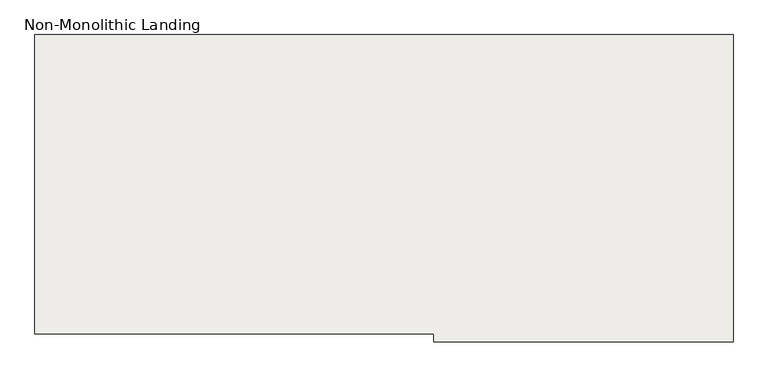
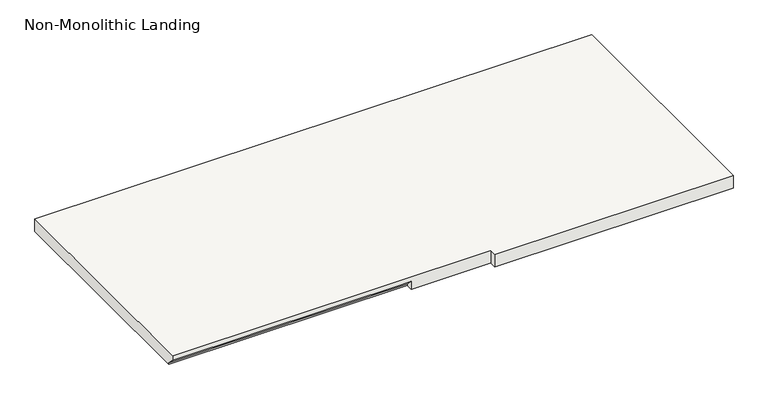
"""IFC4 building model written with IfcOpenShell, lengths in millimetres: slab geometry, Non-Monolithic Landing."""

from ifc_helpers import new_model, si_unit, origin, place, context, project, spatial, faceted_brep, source, transform, mapped, element, save


def non_monolithic_landing_50a26f39(model_context):
    return source(origin(), model_context, "Body", "Brep", [
        faceted_brep([(-3617.4415084, 23194.7216096, 51800.9005799), (-3617.4415084, 23220.1216096, 51775.5005799), (-2703.0415084, 23220.1216096, 51775.5005799), (-2703.0415084, 23194.7216096, 51800.9005799), (-2398.2415084, 23194.7216096, 51819.9505799), (-2398.2415084, 23169.3216096, 51819.9505799), (-1483.8415084, 23169.3216096, 51819.9505799), (-1483.8415084, 23194.7216096, 51819.9505799), (-1483.8415084, 24109.1216096, 51819.9505799), (-3617.4415084, 24109.1216096, 51819.9505799), (-3617.4415084, 23194.7216096, 51819.9505799), (-2703.0415084, 23220.1216096, 51769.1505799), (-3617.4415084, 23220.1216096, 51769.1505799), (-3617.4415084, 24109.1216096, 51769.1505799), (-1483.8415084, 24109.1216096, 51769.1505799), (-1483.8415084, 23194.7216096, 51769.1505799), (-1483.8415084, 23169.3216096, 51769.1505799), (-2398.2415084, 23169.3216096, 51769.1505799), (-2398.2415084, 23194.7216096, 51769.1505799), (-2703.0415084, 23194.7216096, 51769.1505799)], [[[0, 1, 2, 3]], [[4, 5, 6, 7, 8, 9, 10]], [[11, 12, 13, 14, 15, 16, 17, 18, 19]], [[12, 11, 2, 1]], [[11, 19, 3, 2]], [[4, 10, 0, 3, 19, 18]], [[5, 4, 18, 17]], [[6, 5, 17, 16]], [[7, 6, 16, 15]], [[8, 7, 15, 14]], [[9, 8, 14, 13]], [[10, 9, 13, 12, 1, 0]]]),
    ])


if __name__ == "__main__":
    model = new_model("IFC4")
    model_context = context("Model", 3, world=origin())
    ifc_project = project(units=[si_unit("LENGTHUNIT", "METRE", prefix="MILLI")], contexts=[model_context])
    site = spatial("IfcSite", under=ifc_project)
    building = spatial("IfcBuilding", under=site)
    placement = place(None, origin())
    non_monolithic_landing_shape = non_monolithic_landing_50a26f39(model_context)
    element("IfcSlab", 1, ObjectType="Non-Monolithic Landing", at=placement, inside=building, context=model_context, shape_type="MappedRepresentation", body=[
        mapped(non_monolithic_landing_shape, transform((0.0, 0.0, 0.0), x_axis=(1.0, 0.0, 0.0), y_axis=(0.0, 1.0, 0.0), z_axis=(0.0, 0.0, 1.0))),
    ])
    save(model, "model.ifc")
